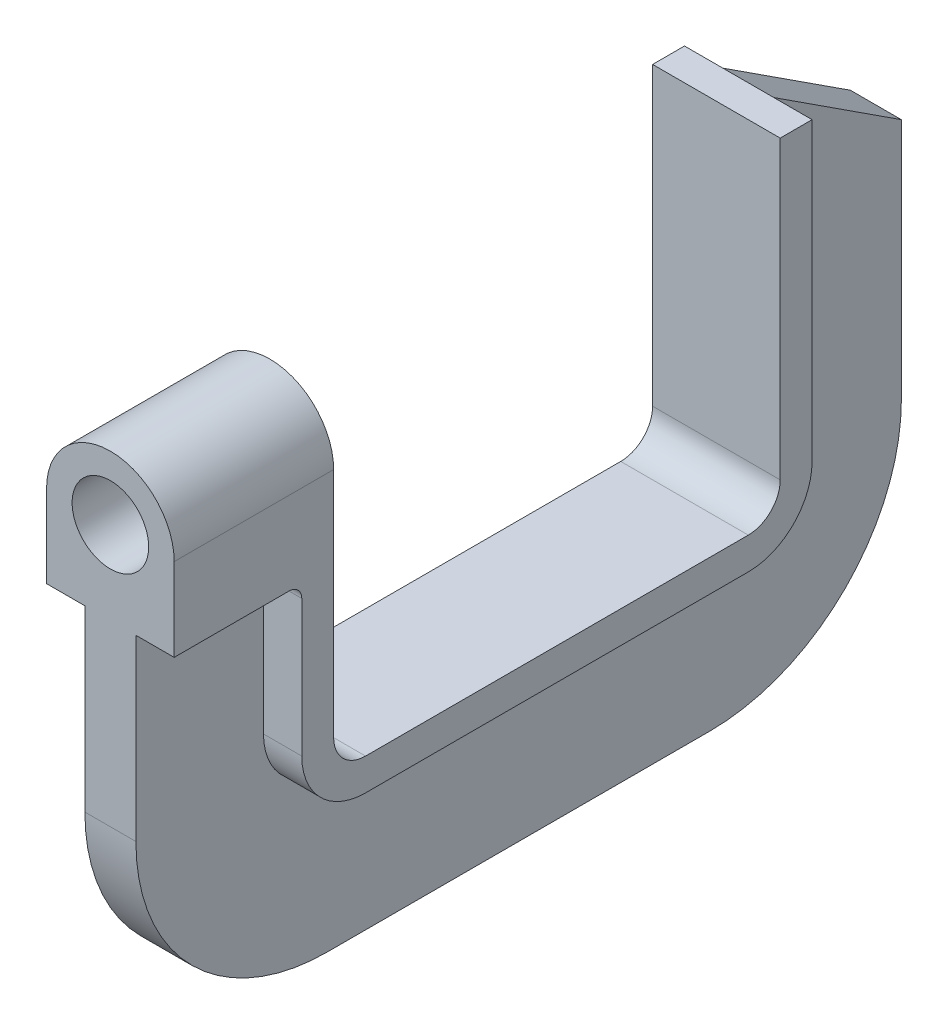
from build123d import *

# Parameters (mm, degrees)
FRAME_PLATE_8MM_DEPTH      = 4
FRAME_RIM_8MM_DEPTH        = 4
FRAME_FLANGE_20MM_DEPTH    = 10
SCREW_BOSS_DEPTH           = 25
RELIEF_CHANNEL_CUT_DEPTH   = 25
M12X1_5_TAPPED_HOLE1_D     = 12
M12X1_5_TAPPED_HOLE1_DEPTH = 25
EDGE_FILLET_R2_R           = 2


with BuildPart() as part:
    # Frame Profile Sketch → Frame Plate 8mm (new, symmetric)
    with BuildSketch(Plane(origin=(0, 0, 0), x_dir=(0, 0, -1), z_dir=(1, 0, 0))):
        with BuildLine():
            ThreePointArc((-65, -81), (-86.213203436, -72.213203436), (-95, -51))
            Line((-95, -51), (-95, 0))
            Line((-95, 0), (-75, 0))
            Line((-75, 0), (-75, -46.399278983))
            ThreePointArc((-75, -46.399278983), (-72.071067812, -53.470346795), (-65, -56.399278983))
            Line((-65, -56.399278983), (-5, -56.399278983))
            ThreePointArc((-5, -56.399278983), (2.071067812, -53.470346795), (5, -46.399278983))
            Line((5, -46.399278983), (5, 0))
            Line((5, 0), (25, -13))
            Line((25, -13), (25, -51))
            ThreePointArc((25, -51), (16.213203436, -72.213203436), (-5, -81))
            Line((-5, -81), (-65, -81))
        make_face()
    extrude(amount=FRAME_PLATE_8MM_DEPTH, both=True)

    # Sketch1_3 → Frame Rim 8mm (add, symmetric)
    with BuildSketch(Plane(origin=(0, 0, 0), x_dir=(0, 0, -1), z_dir=(1, 0, 0))):
        with BuildLine():
            ThreePointArc((-65, -56.399278983), (-72.071067812, -53.470346795), (-75, -46.399278983))
            Line((-75, -46.399278983), (-75, 0))
            Line((-75, 0), (-70, 0))
            Line((-70, 0), (-70, -46.399278983))
            ThreePointArc((-70, -46.399278983), (-68.535533906, -49.934812889), (-65, -51.399278983))
            Line((-65, -51.399278983), (-5, -51.399278983))
            ThreePointArc((-5, -51.399278983), (-1.464466094, -49.934812889), (0, -46.399278983))
            Line((0, -46.399278983), (0, 0))
            Line((0, 0), (5, 0))
            Line((5, 0), (5, -46.399278983))
            ThreePointArc((5, -46.399278983), (2.071067812, -53.470346795), (-5, -56.399278983))
            Line((-5, -56.399278983), (-65, -56.399278983))
        make_face()
    extrude(amount=FRAME_RIM_8MM_DEPTH, both=True)

    # Sketch1_4 → Frame Flange 20mm (add, symmetric)
    with BuildSketch(Plane(origin=(0, 0, 0), x_dir=(0, 0, -1), z_dir=(1, 0, 0))):
        with BuildLine():
            ThreePointArc((-65, -56.399278983), (-72.071067812, -53.470346795), (-75, -46.399278983))
            Line((-75, -46.399278983), (-75, 0))
            Line((-75, 0), (-70, 0))
            Line((-70, 0), (-70, -46.399278983))
            ThreePointArc((-70, -46.399278983), (-68.535533906, -49.934812889), (-65, -51.399278983))
            Line((-65, -51.399278983), (-5, -51.399278983))
            ThreePointArc((-5, -51.399278983), (-1.464466094, -49.934812889), (0, -46.399278983))
            Line((0, -46.399278983), (0, 0))
            Line((0, 0), (5, 0))
            Line((5, 0), (5, -46.399278983))
            ThreePointArc((5, -46.399278983), (2.071067812, -53.470346795), (-5, -56.399278983))
            Line((-5, -56.399278983), (-65, -56.399278983))
        make_face()
    extrude(amount=FRAME_FLANGE_20MM_DEPTH, both=True)

    # Screw Boss Sketch → Screw Boss (add)
    with BuildSketch(Plane.XY.offset(95)):
        with BuildLine():
            Line((-10, -10), (-10, -23))
            Line((-10, -23), (10, -23))
            Line((10, -23), (10, -10))
            ThreePointArc((10, -10), (0, 0), (-10, -10))
        make_face()
    extrude(amount=-SCREW_BOSS_DEPTH)

    # Relief Channel Sketch → Relief Channel Cut (cut)
    with BuildSketch(Plane.XY.offset(95)):
        with BuildLine():
            Line((-10, 0), (-4, 0))
            Line((-4, 0), (-4, -0.83484861))
            ThreePointArc((-4, -0.83484861), (-8.366600265, -4.522774425), (-10, -10))
            Line((-10, -10), (-10, 0))
        make_face()
        with BuildLine():
            Line((-4, 0), (-4, -0.83484861))
            ThreePointArc((-4, -0.83484861), (-2.043096424, -0.210936868), (2.7e-08, 0))
            Line((2.7e-08, 0), (-4, 0))
        make_face()
        with BuildLine():
            Line((4, 0), (2.7e-08, 0))
            ThreePointArc((2.7e-08, 0), (2.04309645, -0.210936873), (4, -0.83484861))
            Line((4, -0.83484861), (4, 0))
        make_face()
        with BuildLine():
            Line((10, -10), (10, 0))
            Line((10, 0), (4, 0))
            Line((4, 0), (4, -0.83484861))
            ThreePointArc((4, -0.83484861), (8.366600265, -4.522774425), (10, -10))
        make_face()
    extrude(amount=-RELIEF_CHANNEL_CUT_DEPTH, mode=Mode.SUBTRACT)

    # M12x1.5 Tapped Hole1
    with Locations(Plane.XY.offset(95)):
        with Locations((0, -10)):
            Hole(M12X1_5_TAPPED_HOLE1_D / 2, depth=M12X1_5_TAPPED_HOLE1_DEPTH)

    # Edge Fillet R2
    edge_fillet_r2_edges = [part.edges().sort_by_distance(p)[0] for p in [
        (-7, -23, 75),
        (7, -23, 75),
    ]]
    fillet(edge_fillet_r2_edges, radius=EDGE_FILLET_R2_R)


solid = part.part
